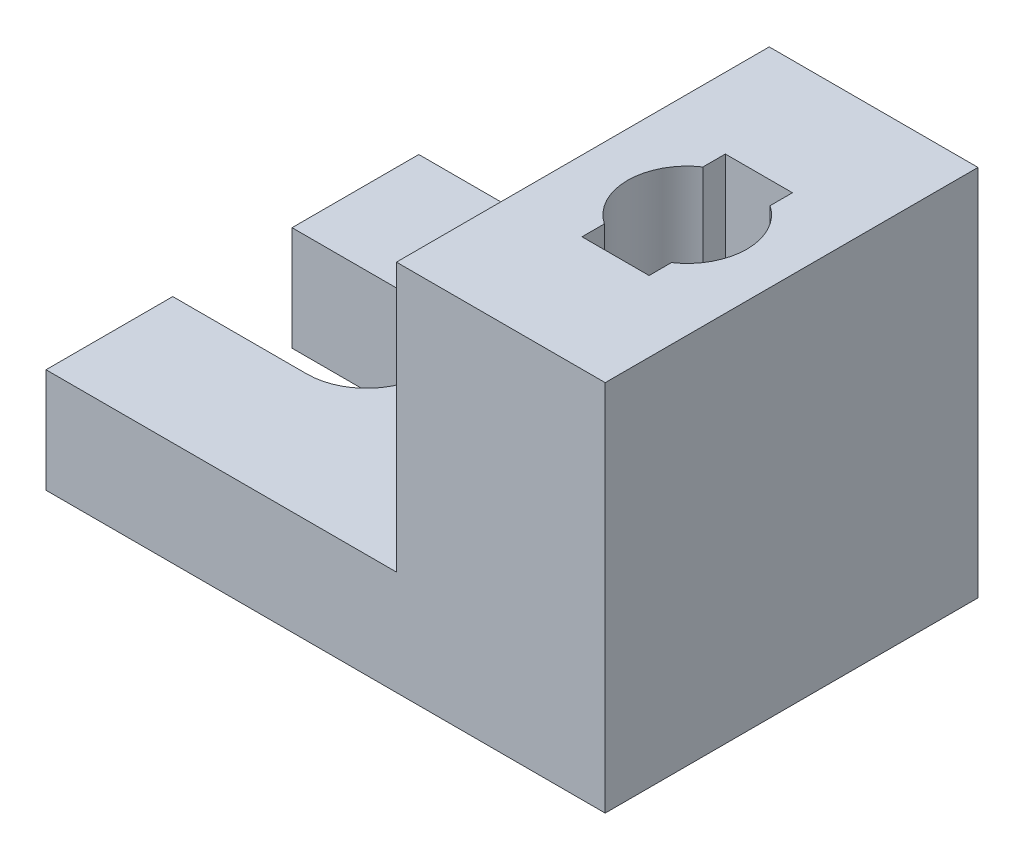
ISO-10303-21;
HEADER;
FILE_DESCRIPTION(('STEP AP214'),'2;1');
FILE_NAME('part.step','',(''),(''),'','','');
FILE_SCHEMA(('AUTOMOTIVE_DESIGN { 1 0 10303 214 1 1 1 1 }'));
ENDSEC;
DATA;
#1=APPLICATION_CONTEXT('core data for automotive mechanical design processes');
#2=APPLICATION_PROTOCOL_DEFINITION('international standard','automotive_design',2000,#1);
#3=PRODUCT_CONTEXT('',#1,'mechanical');
#4=PRODUCT('Part','Part','',(#3));
#5=PRODUCT_RELATED_PRODUCT_CATEGORY('part','',(#4));
#6=PRODUCT_DEFINITION_FORMATION('','',#4);
#7=PRODUCT_DEFINITION_CONTEXT('part definition',#1,'design');
#8=PRODUCT_DEFINITION('design','',#6,#7);
#9=PRODUCT_DEFINITION_SHAPE('','',#8);
#10=(LENGTH_UNIT() NAMED_UNIT(*) SI_UNIT(.MILLI.,.METRE.));
#11=(NAMED_UNIT(*) PLANE_ANGLE_UNIT() SI_UNIT($,.RADIAN.));
#12=(NAMED_UNIT(*) SI_UNIT($,.STERADIAN.) SOLID_ANGLE_UNIT());
#13=UNCERTAINTY_MEASURE_WITH_UNIT(LENGTH_MEASURE(1.E-05),#10,'distance_accuracy_value','');
#14=(GEOMETRIC_REPRESENTATION_CONTEXT(3) GLOBAL_UNCERTAINTY_ASSIGNED_CONTEXT((#13)) GLOBAL_UNIT_ASSIGNED_CONTEXT((#10,
#11,#12)) REPRESENTATION_CONTEXT('',''));
#15=CARTESIAN_POINT('',(0.,0.,0.));
#16=DIRECTION('',(0.,0.,1.));
#17=DIRECTION('',(1.,0.,0.));
#18=AXIS2_PLACEMENT_3D('',#15,#16,#17);
#19=CARTESIAN_POINT('',(0.,0.,100.));
#20=DIRECTION('',(1.,0.,0.));
#21=DIRECTION('',(0.,0.,-1.));
#22=AXIS2_PLACEMENT_3D('',#19,#20,#21);
#23=PLANE('',#22);
#24=DIRECTION('',(0.,0.,-1.));
#25=VECTOR('',#24,1.);
#26=CARTESIAN_POINT('',(0.,28.,100.));
#27=LINE('',#26,#25);
#28=CARTESIAN_POINT('',(0.,28.,100.));
#29=VERTEX_POINT('',#28);
#30=CARTESIAN_POINT('',(0.,28.,66.));
#31=VERTEX_POINT('',#30);
#32=EDGE_CURVE('E335',#29,#31,#27,.T.);
#33=ORIENTED_EDGE('',*,*,#32,.T.);
#34=DIRECTION('',(0.,1.,0.));
#35=VECTOR('',#34,1.);
#36=CARTESIAN_POINT('',(0.,0.,66.));
#37=LINE('',#36,#35);
#38=CARTESIAN_POINT('',(0.,0.,66.));
#39=VERTEX_POINT('',#38);
#40=EDGE_CURVE('E217',#39,#31,#37,.T.);
#41=ORIENTED_EDGE('',*,*,#40,.F.);
#42=DIRECTION('',(0.,0.,-1.));
#43=VECTOR('',#42,1.);
#44=CARTESIAN_POINT('',(0.,0.,100.));
#45=LINE('',#44,#43);
#46=CARTESIAN_POINT('',(0.,0.,100.));
#47=VERTEX_POINT('',#46);
#48=EDGE_CURVE('E11',#47,#39,#45,.T.);
#49=ORIENTED_EDGE('',*,*,#48,.F.);
#50=DIRECTION('',(0.,-1.,0.));
#51=VECTOR('',#50,1.);
#52=CARTESIAN_POINT('',(0.,0.,100.));
#53=LINE('',#52,#51);
#54=EDGE_CURVE('E310',#29,#47,#53,.T.);
#55=ORIENTED_EDGE('',*,*,#54,.F.);
#56=EDGE_LOOP('',(#33,#41,#49,#55));
#57=FACE_BOUND('',#56,.T.);
#58=ADVANCED_FACE('F44',(#57),#23,.F.);
#59=CARTESIAN_POINT('',(56.,28.,40.));
#60=DIRECTION('',(-0.784045824461761,0.620702944365561,0.));
#61=DIRECTION('',(-0.620702944365561,-0.784045824461761,0.));
#62=AXIS2_PLACEMENT_3D('',#59,#60,#61);
#63=PLANE('',#62);
#64=DIRECTION('',(0.620702944365561,0.784045824461761,0.));
#65=VECTOR('',#64,1.);
#66=CARTESIAN_POINT('',(56.,28.,44.));
#67=LINE('',#66,#65);
#68=CARTESIAN_POINT('',(56.,28.,44.));
#69=VERTEX_POINT('',#68);
#70=CARTESIAN_POINT('',(94.,76.,44.));
#71=VERTEX_POINT('',#70);
#72=EDGE_CURVE('E220',#69,#71,#67,.T.);
#73=ORIENTED_EDGE('',*,*,#72,.F.);
#74=DIRECTION('',(0.,0.,1.));
#75=VECTOR('',#74,1.);
#76=CARTESIAN_POINT('',(56.,28.,40.));
#77=LINE('',#76,#75);
#78=CARTESIAN_POINT('',(56.,28.,56.));
#79=VERTEX_POINT('',#78);
#80=EDGE_CURVE('E237',#69,#79,#77,.T.);
#81=ORIENTED_EDGE('',*,*,#80,.T.);
#82=DIRECTION('',(-0.620702944365561,-0.784045824461761,0.));
#83=VECTOR('',#82,1.);
#84=CARTESIAN_POINT('',(56.,28.,56.));
#85=LINE('',#84,#83);
#86=CARTESIAN_POINT('',(94.,76.,56.));
#87=VERTEX_POINT('',#86);
#88=EDGE_CURVE('E226',#87,#79,#85,.T.);
#89=ORIENTED_EDGE('',*,*,#88,.F.);
#90=DIRECTION('',(0.,0.,1.));
#91=VECTOR('',#90,1.);
#92=CARTESIAN_POINT('',(94.,76.,40.));
#93=LINE('',#92,#91);
#94=EDGE_CURVE('E67',#71,#87,#93,.T.);
#95=ORIENTED_EDGE('',*,*,#94,.F.);
#96=EDGE_LOOP('',(#73,#81,#89,#95));
#97=FACE_BOUND('',#96,.T.);
#98=ADVANCED_FACE('F389',(#97),#63,.T.);
#99=CARTESIAN_POINT('',(0.,0.,34.));
#100=VERTEX_POINT('',#99);
#101=CARTESIAN_POINT('',(0.,0.,0.));
#102=VERTEX_POINT('',#101);
#103=EDGE_CURVE('E52',#100,#102,#45,.T.);
#104=ORIENTED_EDGE('',*,*,#103,.F.);
#105=DIRECTION('',(0.,1.,0.));
#106=VECTOR('',#105,1.);
#107=CARTESIAN_POINT('',(0.,0.,34.));
#108=LINE('',#107,#106);
#109=CARTESIAN_POINT('',(0.,28.,34.));
#110=VERTEX_POINT('',#109);
#111=EDGE_CURVE('E193',#100,#110,#108,.T.);
#112=ORIENTED_EDGE('',*,*,#111,.T.);
#113=CARTESIAN_POINT('',(0.,28.,0.));
#114=VERTEX_POINT('',#113);
#115=EDGE_CURVE('E322',#110,#114,#27,.T.);
#116=ORIENTED_EDGE('',*,*,#115,.T.);
#117=DIRECTION('',(0.,-1.,0.));
#118=VECTOR('',#117,1.);
#119=CARTESIAN_POINT('',(0.,0.,0.));
#120=LINE('',#119,#118);
#121=EDGE_CURVE('E292',#114,#102,#120,.T.);
#122=ORIENTED_EDGE('',*,*,#121,.T.);
#123=EDGE_LOOP('',(#104,#112,#116,#122));
#124=FACE_BOUND('',#123,.T.);
#125=ADVANCED_FACE('F50',(#124),#23,.F.);
#126=CARTESIAN_POINT('',(0.,0.,100.));
#127=DIRECTION('',(0.,1.,0.));
#128=DIRECTION('',(0.,0.,1.));
#129=AXIS2_PLACEMENT_3D('',#126,#127,#128);
#130=PLANE('',#129);
#131=ORIENTED_EDGE('',*,*,#48,.T.);
#132=DIRECTION('',(1.,0.,0.));
#133=VECTOR('',#132,1.);
#134=CARTESIAN_POINT('',(36.,0.,66.));
#135=LINE('',#134,#133);
#136=CARTESIAN_POINT('',(36.,0.,66.));
#137=VERTEX_POINT('',#136);
#138=EDGE_CURVE('E196',#39,#137,#135,.T.);
#139=ORIENTED_EDGE('',*,*,#138,.T.);
#140=CARTESIAN_POINT('',(36.,0.,50.));
#141=DIRECTION('',(0.,1.,0.));
#142=DIRECTION('',(0.,0.,1.));
#143=AXIS2_PLACEMENT_3D('',#140,#141,#142);
#144=CIRCLE('',#143,16.);
#145=CARTESIAN_POINT('',(36.,0.,34.));
#146=VERTEX_POINT('',#145);
#147=EDGE_CURVE('E192',#137,#146,#144,.T.);
#148=ORIENTED_EDGE('',*,*,#147,.T.);
#149=DIRECTION('',(-1.,0.,0.));
#150=VECTOR('',#149,1.);
#151=CARTESIAN_POINT('',(36.,0.,34.));
#152=LINE('',#151,#150);
#153=EDGE_CURVE('E198',#146,#100,#152,.T.);
#154=ORIENTED_EDGE('',*,*,#153,.T.);
#155=ORIENTED_EDGE('',*,*,#103,.T.);
#156=DIRECTION('',(1.,0.,0.));
#157=VECTOR('',#156,1.);
#158=CARTESIAN_POINT('',(0.,0.,0.));
#159=LINE('',#158,#157);
#160=CARTESIAN_POINT('',(150.,0.,0.));
#161=VERTEX_POINT('',#160);
#162=EDGE_CURVE('E321',#102,#161,#159,.T.);
#163=ORIENTED_EDGE('',*,*,#162,.T.);
#164=DIRECTION('',(0.,0.,-1.));
#165=VECTOR('',#164,1.);
#166=CARTESIAN_POINT('',(150.,0.,100.));
#167=LINE('',#166,#165);
#168=CARTESIAN_POINT('',(150.,0.,100.));
#169=VERTEX_POINT('',#168);
#170=EDGE_CURVE('E343',#169,#161,#167,.T.);
#171=ORIENTED_EDGE('',*,*,#170,.F.);
#172=DIRECTION('',(1.,0.,0.));
#173=VECTOR('',#172,1.);
#174=CARTESIAN_POINT('',(0.,0.,100.));
#175=LINE('',#174,#173);
#176=EDGE_CURVE('E309',#47,#169,#175,.T.);
#177=ORIENTED_EDGE('',*,*,#176,.F.);
#178=EDGE_LOOP('',(#131,#139,#148,#154,#155,#163,#171,#177));
#179=FACE_BOUND('',#178,.T.);
#180=ADVANCED_FACE('F205',(#179),#130,.F.);
#181=CARTESIAN_POINT('',(150.,0.,100.));
#182=DIRECTION('',(-1.,0.,0.));
#183=DIRECTION('',(0.,0.,1.));
#184=AXIS2_PLACEMENT_3D('',#181,#182,#183);
#185=PLANE('',#184);
#186=DIRECTION('',(0.,1.,0.));
#187=VECTOR('',#186,1.);
#188=CARTESIAN_POINT('',(150.,0.,0.));
#189=LINE('',#188,#187);
#190=CARTESIAN_POINT('',(150.,100.,0.));
#191=VERTEX_POINT('',#190);
#192=EDGE_CURVE('E326',#161,#191,#189,.T.);
#193=ORIENTED_EDGE('',*,*,#192,.T.);
#194=DIRECTION('',(0.,0.,-1.));
#195=VECTOR('',#194,1.);
#196=CARTESIAN_POINT('',(150.,100.,100.));
#197=LINE('',#196,#195);
#198=CARTESIAN_POINT('',(150.,100.,100.));
#199=VERTEX_POINT('',#198);
#200=EDGE_CURVE('E344',#199,#191,#197,.T.);
#201=ORIENTED_EDGE('',*,*,#200,.F.);
#202=DIRECTION('',(0.,1.,0.));
#203=VECTOR('',#202,1.);
#204=CARTESIAN_POINT('',(150.,0.,100.));
#205=LINE('',#204,#203);
#206=EDGE_CURVE('E312',#169,#199,#205,.T.);
#207=ORIENTED_EDGE('',*,*,#206,.F.);
#208=ORIENTED_EDGE('',*,*,#170,.T.);
#209=EDGE_LOOP('',(#193,#201,#207,#208));
#210=FACE_BOUND('',#209,.T.);
#211=ADVANCED_FACE('F369',(#210),#185,.F.);
#212=CARTESIAN_POINT('',(150.,100.,100.));
#213=DIRECTION('',(0.,-1.,0.));
#214=DIRECTION('',(0.,0.,-1.));
#215=AXIS2_PLACEMENT_3D('',#212,#213,#214);
#216=PLANE('',#215);
#217=DIRECTION('',(0.,0.,-1.));
#218=VECTOR('',#217,1.);
#219=CARTESIAN_POINT('',(131.,100.,30.7712434446771));
#220=LINE('',#219,#218);
#221=CARTESIAN_POINT('',(131.,100.,36.7712434446771));
#222=VERTEX_POINT('',#221);
#223=CARTESIAN_POINT('',(131.,100.,30.7712434446771));
#224=VERTEX_POINT('',#223);
#225=EDGE_CURVE('E270',#222,#224,#220,.T.);
#226=ORIENTED_EDGE('',*,*,#225,.F.);
#227=CARTESIAN_POINT('',(122.,100.,50.));
#228=DIRECTION('',(0.,1.,0.));
#229=DIRECTION('',(0.,0.,1.));
#230=AXIS2_PLACEMENT_3D('',#227,#228,#229);
#231=CIRCLE('',#230,16.);
#232=CARTESIAN_POINT('',(131.,100.,63.2287565553229));
#233=VERTEX_POINT('',#232);
#234=EDGE_CURVE('E241',#233,#222,#231,.T.);
#235=ORIENTED_EDGE('',*,*,#234,.F.);
#236=DIRECTION('',(0.,0.,-1.));
#237=VECTOR('',#236,1.);
#238=CARTESIAN_POINT('',(131.,100.,63.2287565553229));
#239=LINE('',#238,#237);
#240=CARTESIAN_POINT('',(131.,100.,69.2287565553229));
#241=VERTEX_POINT('',#240);
#242=EDGE_CURVE('E250',#241,#233,#239,.T.);
#243=ORIENTED_EDGE('',*,*,#242,.F.);
#244=DIRECTION('',(1.,0.,0.));
#245=VECTOR('',#244,1.);
#246=CARTESIAN_POINT('',(113.,100.,69.228756555323));
#247=LINE('',#246,#245);
#248=CARTESIAN_POINT('',(113.,100.,69.228756555323));
#249=VERTEX_POINT('',#248);
#250=EDGE_CURVE('E284',#249,#241,#247,.T.);
#251=ORIENTED_EDGE('',*,*,#250,.F.);
#252=DIRECTION('',(0.,0.,1.));
#253=VECTOR('',#252,1.);
#254=CARTESIAN_POINT('',(113.,100.,63.228756555323));
#255=LINE('',#254,#253);
#256=CARTESIAN_POINT('',(113.,100.,63.228756555323));
#257=VERTEX_POINT('',#256);
#258=EDGE_CURVE('E285',#257,#249,#255,.T.);
#259=ORIENTED_EDGE('',*,*,#258,.F.);
#260=CARTESIAN_POINT('',(122.,100.,50.));
#261=DIRECTION('',(0.,1.,0.));
#262=DIRECTION('',(0.,0.,1.));
#263=AXIS2_PLACEMENT_3D('',#260,#261,#262);
#264=CIRCLE('',#263,16.);
#265=CARTESIAN_POINT('',(113.,100.,36.7712434446771));
#266=VERTEX_POINT('',#265);
#267=EDGE_CURVE('E276',#266,#257,#264,.T.);
#268=ORIENTED_EDGE('',*,*,#267,.F.);
#269=DIRECTION('',(0.,0.,1.));
#270=VECTOR('',#269,1.);
#271=CARTESIAN_POINT('',(113.,100.,30.7712434446771));
#272=LINE('',#271,#270);
#273=CARTESIAN_POINT('',(113.,100.,30.7712434446771));
#274=VERTEX_POINT('',#273);
#275=EDGE_CURVE('E277',#274,#266,#272,.T.);
#276=ORIENTED_EDGE('',*,*,#275,.F.);
#277=DIRECTION('',(-1.,0.,0.));
#278=VECTOR('',#277,1.);
#279=CARTESIAN_POINT('',(113.,100.,30.7712434446771));
#280=LINE('',#279,#278);
#281=EDGE_CURVE('E271',#224,#274,#280,.T.);
#282=ORIENTED_EDGE('',*,*,#281,.F.);
#283=EDGE_LOOP('',(#226,#235,#243,#251,#259,#268,#276,#282));
#284=FACE_BOUND('',#283,.T.);
#285=DIRECTION('',(-1.,0.,0.));
#286=VECTOR('',#285,1.);
#287=CARTESIAN_POINT('',(150.,100.,0.));
#288=LINE('',#287,#286);
#289=CARTESIAN_POINT('',(94.,100.,0.));
#290=VERTEX_POINT('',#289);
#291=EDGE_CURVE('E327',#191,#290,#288,.T.);
#292=ORIENTED_EDGE('',*,*,#291,.T.);
#293=DIRECTION('',(0.,0.,-1.));
#294=VECTOR('',#293,1.);
#295=CARTESIAN_POINT('',(94.,100.,100.));
#296=LINE('',#295,#294);
#297=CARTESIAN_POINT('',(94.,100.,100.));
#298=VERTEX_POINT('',#297);
#299=EDGE_CURVE('E338',#298,#290,#296,.T.);
#300=ORIENTED_EDGE('',*,*,#299,.F.);
#301=DIRECTION('',(-1.,0.,0.));
#302=VECTOR('',#301,1.);
#303=CARTESIAN_POINT('',(150.,100.,100.));
#304=LINE('',#303,#302);
#305=EDGE_CURVE('E314',#199,#298,#304,.T.);
#306=ORIENTED_EDGE('',*,*,#305,.F.);
#307=ORIENTED_EDGE('',*,*,#200,.T.);
#308=EDGE_LOOP('',(#292,#300,#306,#307));
#309=FACE_BOUND('',#308,.T.);
#310=ADVANCED_FACE('F368',(#284,#309),#216,.F.);
#311=CARTESIAN_POINT('',(94.,28.,100.));
#312=DIRECTION('',(1.,0.,0.));
#313=DIRECTION('',(0.,0.,-1.));
#314=AXIS2_PLACEMENT_3D('',#311,#312,#313);
#315=PLANE('',#314);
#316=DIRECTION('',(0.,-1.,0.));
#317=VECTOR('',#316,1.);
#318=CARTESIAN_POINT('',(94.,76.,44.));
#319=LINE('',#318,#317);
#320=CARTESIAN_POINT('',(94.,28.,44.));
#321=VERTEX_POINT('',#320);
#322=EDGE_CURVE('E224',#71,#321,#319,.T.);
#323=ORIENTED_EDGE('',*,*,#322,.F.);
#324=ORIENTED_EDGE('',*,*,#94,.T.);
#325=DIRECTION('',(0.,1.,0.));
#326=VECTOR('',#325,1.);
#327=CARTESIAN_POINT('',(94.,76.,56.));
#328=LINE('',#327,#326);
#329=CARTESIAN_POINT('',(94.,28.,56.));
#330=VERTEX_POINT('',#329);
#331=EDGE_CURVE('E234',#330,#87,#328,.T.);
#332=ORIENTED_EDGE('',*,*,#331,.F.);
#333=DIRECTION('',(0.,0.,1.));
#334=VECTOR('',#333,1.);
#335=CARTESIAN_POINT('',(94.,28.,56.));
#336=LINE('',#335,#334);
#337=CARTESIAN_POINT('',(94.,28.,100.));
#338=VERTEX_POINT('',#337);
#339=EDGE_CURVE('E236',#330,#338,#336,.T.);
#340=ORIENTED_EDGE('',*,*,#339,.T.);
#341=DIRECTION('',(0.,-1.,0.));
#342=VECTOR('',#341,1.);
#343=CARTESIAN_POINT('',(94.,28.,100.));
#344=LINE('',#343,#342);
#345=EDGE_CURVE('E320',#298,#338,#344,.T.);
#346=ORIENTED_EDGE('',*,*,#345,.F.);
#347=ORIENTED_EDGE('',*,*,#299,.T.);
#348=DIRECTION('',(0.,-1.,0.));
#349=VECTOR('',#348,1.);
#350=CARTESIAN_POINT('',(94.,28.,0.));
#351=LINE('',#350,#349);
#352=CARTESIAN_POINT('',(94.,28.,0.));
#353=VERTEX_POINT('',#352);
#354=EDGE_CURVE('E329',#290,#353,#351,.T.);
#355=ORIENTED_EDGE('',*,*,#354,.T.);
#356=DIRECTION('',(0.,0.,-1.));
#357=VECTOR('',#356,1.);
#358=CARTESIAN_POINT('',(94.,28.,100.));
#359=LINE('',#358,#357);
#360=EDGE_CURVE('E336',#321,#353,#359,.T.);
#361=ORIENTED_EDGE('',*,*,#360,.F.);
#362=EDGE_LOOP('',(#323,#324,#332,#340,#346,#347,#355,#361));
#363=FACE_BOUND('',#362,.T.);
#364=ADVANCED_FACE('F361',(#363),#315,.F.);
#365=CARTESIAN_POINT('',(0.,28.,100.));
#366=DIRECTION('',(0.,-1.,0.));
#367=DIRECTION('',(0.,0.,-1.));
#368=AXIS2_PLACEMENT_3D('',#365,#366,#367);
#369=PLANE('',#368);
#370=CARTESIAN_POINT('',(36.,28.,50.));
#371=DIRECTION('',(0.,1.,0.));
#372=DIRECTION('',(0.,0.,1.));
#373=AXIS2_PLACEMENT_3D('',#370,#371,#372);
#374=CIRCLE('',#373,16.);
#375=CARTESIAN_POINT('',(36.,28.,66.));
#376=VERTEX_POINT('',#375);
#377=CARTESIAN_POINT('',(36.,28.,34.));
#378=VERTEX_POINT('',#377);
#379=EDGE_CURVE('E58',#376,#378,#374,.T.);
#380=ORIENTED_EDGE('',*,*,#379,.F.);
#381=DIRECTION('',(1.,0.,0.));
#382=VECTOR('',#381,1.);
#383=CARTESIAN_POINT('',(36.,28.,66.));
#384=LINE('',#383,#382);
#385=EDGE_CURVE('E207',#31,#376,#384,.T.);
#386=ORIENTED_EDGE('',*,*,#385,.F.);
#387=ORIENTED_EDGE('',*,*,#32,.F.);
#388=DIRECTION('',(-1.,0.,0.));
#389=VECTOR('',#388,1.);
#390=CARTESIAN_POINT('',(0.,28.,100.));
#391=LINE('',#390,#389);
#392=EDGE_CURVE('E316',#338,#29,#391,.T.);
#393=ORIENTED_EDGE('',*,*,#392,.F.);
#394=ORIENTED_EDGE('',*,*,#339,.F.);
#395=DIRECTION('',(1.,0.,0.));
#396=VECTOR('',#395,1.);
#397=CARTESIAN_POINT('',(94.,28.,56.));
#398=LINE('',#397,#396);
#399=EDGE_CURVE('E233',#79,#330,#398,.T.);
#400=ORIENTED_EDGE('',*,*,#399,.F.);
#401=ORIENTED_EDGE('',*,*,#80,.F.);
#402=DIRECTION('',(-1.,0.,0.));
#403=VECTOR('',#402,1.);
#404=CARTESIAN_POINT('',(94.,28.,44.));
#405=LINE('',#404,#403);
#406=EDGE_CURVE('E228',#321,#69,#405,.T.);
#407=ORIENTED_EDGE('',*,*,#406,.F.);
#408=ORIENTED_EDGE('',*,*,#360,.T.);
#409=DIRECTION('',(-1.,0.,0.));
#410=VECTOR('',#409,1.);
#411=CARTESIAN_POINT('',(0.,28.,0.));
#412=LINE('',#411,#410);
#413=EDGE_CURVE('E311',#353,#114,#412,.T.);
#414=ORIENTED_EDGE('',*,*,#413,.T.);
#415=ORIENTED_EDGE('',*,*,#115,.F.);
#416=DIRECTION('',(-1.,0.,0.));
#417=VECTOR('',#416,1.);
#418=CARTESIAN_POINT('',(36.,28.,34.));
#419=LINE('',#418,#417);
#420=EDGE_CURVE('E209',#378,#110,#419,.T.);
#421=ORIENTED_EDGE('',*,*,#420,.F.);
#422=EDGE_LOOP('',(#380,#386,#387,#393,#394,#400,#401,#407,#408,#414,#415,#421));
#423=FACE_BOUND('',#422,.T.);
#424=ADVANCED_FACE('F359',(#423),#369,.F.);
#425=CARTESIAN_POINT('',(0.,0.,100.));
#426=DIRECTION('',(0.,0.,-1.));
#427=DIRECTION('',(-1.,0.,0.));
#428=AXIS2_PLACEMENT_3D('',#425,#426,#427);
#429=PLANE('',#428);
#430=ORIENTED_EDGE('',*,*,#345,.T.);
#431=ORIENTED_EDGE('',*,*,#392,.T.);
#432=ORIENTED_EDGE('',*,*,#54,.T.);
#433=ORIENTED_EDGE('',*,*,#176,.T.);
#434=ORIENTED_EDGE('',*,*,#206,.T.);
#435=ORIENTED_EDGE('',*,*,#305,.T.);
#436=EDGE_LOOP('',(#430,#431,#432,#433,#434,#435));
#437=FACE_BOUND('',#436,.T.);
#438=ADVANCED_FACE('F375',(#437),#429,.F.);
#439=CARTESIAN_POINT('',(0.,0.,0.));
#440=DIRECTION('',(0.,0.,-1.));
#441=DIRECTION('',(-1.,0.,0.));
#442=AXIS2_PLACEMENT_3D('',#439,#440,#441);
#443=PLANE('',#442);
#444=ORIENTED_EDGE('',*,*,#121,.F.);
#445=ORIENTED_EDGE('',*,*,#413,.F.);
#446=ORIENTED_EDGE('',*,*,#354,.F.);
#447=ORIENTED_EDGE('',*,*,#291,.F.);
#448=ORIENTED_EDGE('',*,*,#192,.F.);
#449=ORIENTED_EDGE('',*,*,#162,.F.);
#450=EDGE_LOOP('',(#444,#445,#446,#447,#448,#449));
#451=FACE_BOUND('',#450,.T.);
#452=ADVANCED_FACE('F355',(#451),#443,.T.);
#453=CARTESIAN_POINT('',(122.,50.,50.));
#454=DIRECTION('',(0.,1.,0.));
#455=DIRECTION('',(0.,0.,1.));
#456=AXIS2_PLACEMENT_3D('',#453,#454,#455);
#457=CYLINDRICAL_SURFACE('',#456,16.);
#458=ORIENTED_EDGE('',*,*,#234,.T.);
#459=DIRECTION('',(0.,1.,0.));
#460=VECTOR('',#459,1.);
#461=CARTESIAN_POINT('',(131.,50.,36.7712434446771));
#462=LINE('',#461,#460);
#463=CARTESIAN_POINT('',(131.,50.,36.7712434446771));
#464=VERTEX_POINT('',#463);
#465=EDGE_CURVE('E269',#464,#222,#462,.T.);
#466=ORIENTED_EDGE('',*,*,#465,.F.);
#467=CARTESIAN_POINT('',(122.,50.,50.));
#468=DIRECTION('',(0.,1.,0.));
#469=DIRECTION('',(0.,0.,1.));
#470=AXIS2_PLACEMENT_3D('',#467,#468,#469);
#471=CIRCLE('',#470,16.);
#472=CARTESIAN_POINT('',(131.,50.,63.2287565553229));
#473=VERTEX_POINT('',#472);
#474=EDGE_CURVE('E243',#473,#464,#471,.T.);
#475=ORIENTED_EDGE('',*,*,#474,.F.);
#476=DIRECTION('',(0.,1.,0.));
#477=VECTOR('',#476,1.);
#478=CARTESIAN_POINT('',(131.,50.,63.2287565553229));
#479=LINE('',#478,#477);
#480=EDGE_CURVE('E290',#473,#233,#479,.T.);
#481=ORIENTED_EDGE('',*,*,#480,.T.);
#482=EDGE_LOOP('',(#458,#466,#475,#481));
#483=FACE_BOUND('',#482,.T.);
#484=ADVANCED_FACE('F424',(#483),#457,.F.);
#485=CARTESIAN_POINT('',(131.,50.,63.2287565553229));
#486=DIRECTION('',(1.,0.,0.));
#487=DIRECTION('',(0.,0.,-1.));
#488=AXIS2_PLACEMENT_3D('',#485,#486,#487);
#489=PLANE('',#488);
#490=ORIENTED_EDGE('',*,*,#242,.T.);
#491=ORIENTED_EDGE('',*,*,#480,.F.);
#492=DIRECTION('',(0.,0.,-1.));
#493=VECTOR('',#492,1.);
#494=CARTESIAN_POINT('',(131.,50.,63.2287565553229));
#495=LINE('',#494,#493);
#496=CARTESIAN_POINT('',(131.,50.,69.2287565553229));
#497=VERTEX_POINT('',#496);
#498=EDGE_CURVE('E264',#497,#473,#495,.T.);
#499=ORIENTED_EDGE('',*,*,#498,.F.);
#500=DIRECTION('',(0.,1.,0.));
#501=VECTOR('',#500,1.);
#502=CARTESIAN_POINT('',(131.,50.,69.2287565553229));
#503=LINE('',#502,#501);
#504=EDGE_CURVE('E291',#497,#241,#503,.T.);
#505=ORIENTED_EDGE('',*,*,#504,.T.);
#506=EDGE_LOOP('',(#490,#491,#499,#505));
#507=FACE_BOUND('',#506,.T.);
#508=ADVANCED_FACE('F427',(#507),#489,.F.);
#509=CARTESIAN_POINT('',(113.,50.,69.228756555323));
#510=DIRECTION('',(0.,0.,1.));
#511=DIRECTION('',(1.,0.,0.));
#512=AXIS2_PLACEMENT_3D('',#509,#510,#511);
#513=PLANE('',#512);
#514=ORIENTED_EDGE('',*,*,#250,.T.);
#515=ORIENTED_EDGE('',*,*,#504,.F.);
#516=DIRECTION('',(1.,0.,0.));
#517=VECTOR('',#516,1.);
#518=CARTESIAN_POINT('',(113.,50.,69.228756555323));
#519=LINE('',#518,#517);
#520=CARTESIAN_POINT('',(113.,50.,69.228756555323));
#521=VERTEX_POINT('',#520);
#522=EDGE_CURVE('E265',#521,#497,#519,.T.);
#523=ORIENTED_EDGE('',*,*,#522,.F.);
#524=DIRECTION('',(0.,1.,0.));
#525=VECTOR('',#524,1.);
#526=CARTESIAN_POINT('',(113.,50.,69.228756555323));
#527=LINE('',#526,#525);
#528=EDGE_CURVE('E294',#521,#249,#527,.T.);
#529=ORIENTED_EDGE('',*,*,#528,.T.);
#530=EDGE_LOOP('',(#514,#515,#523,#529));
#531=FACE_BOUND('',#530,.T.);
#532=ADVANCED_FACE('F452',(#531),#513,.F.);
#533=CARTESIAN_POINT('',(113.,50.,63.228756555323));
#534=DIRECTION('',(-1.,0.,0.));
#535=DIRECTION('',(0.,0.,1.));
#536=AXIS2_PLACEMENT_3D('',#533,#534,#535);
#537=PLANE('',#536);
#538=ORIENTED_EDGE('',*,*,#258,.T.);
#539=ORIENTED_EDGE('',*,*,#528,.F.);
#540=DIRECTION('',(0.,0.,1.));
#541=VECTOR('',#540,1.);
#542=CARTESIAN_POINT('',(113.,50.,63.228756555323));
#543=LINE('',#542,#541);
#544=CARTESIAN_POINT('',(113.,50.,63.228756555323));
#545=VERTEX_POINT('',#544);
#546=EDGE_CURVE('E256',#545,#521,#543,.T.);
#547=ORIENTED_EDGE('',*,*,#546,.F.);
#548=DIRECTION('',(0.,1.,0.));
#549=VECTOR('',#548,1.);
#550=CARTESIAN_POINT('',(113.,50.,63.228756555323));
#551=LINE('',#550,#549);
#552=EDGE_CURVE('E300',#545,#257,#551,.T.);
#553=ORIENTED_EDGE('',*,*,#552,.T.);
#554=EDGE_LOOP('',(#538,#539,#547,#553));
#555=FACE_BOUND('',#554,.T.);
#556=ADVANCED_FACE('F450',(#555),#537,.F.);
#557=CARTESIAN_POINT('',(122.,50.,50.));
#558=DIRECTION('',(0.,1.,0.));
#559=DIRECTION('',(0.,0.,1.));
#560=AXIS2_PLACEMENT_3D('',#557,#558,#559);
#561=CYLINDRICAL_SURFACE('',#560,16.);
#562=ORIENTED_EDGE('',*,*,#267,.T.);
#563=ORIENTED_EDGE('',*,*,#552,.F.);
#564=CARTESIAN_POINT('',(122.,50.,50.));
#565=DIRECTION('',(0.,1.,0.));
#566=DIRECTION('',(0.,0.,1.));
#567=AXIS2_PLACEMENT_3D('',#564,#565,#566);
#568=CIRCLE('',#567,16.);
#569=CARTESIAN_POINT('',(113.,50.,36.7712434446771));
#570=VERTEX_POINT('',#569);
#571=EDGE_CURVE('E257',#570,#545,#568,.T.);
#572=ORIENTED_EDGE('',*,*,#571,.F.);
#573=DIRECTION('',(0.,1.,0.));
#574=VECTOR('',#573,1.);
#575=CARTESIAN_POINT('',(113.,50.,36.7712434446771));
#576=LINE('',#575,#574);
#577=EDGE_CURVE('E299',#570,#266,#576,.T.);
#578=ORIENTED_EDGE('',*,*,#577,.T.);
#579=EDGE_LOOP('',(#562,#563,#572,#578));
#580=FACE_BOUND('',#579,.T.);
#581=ADVANCED_FACE('F442',(#580),#561,.F.);
#582=CARTESIAN_POINT('',(113.,50.,30.7712434446771));
#583=DIRECTION('',(-1.,0.,0.));
#584=DIRECTION('',(0.,0.,1.));
#585=AXIS2_PLACEMENT_3D('',#582,#583,#584);
#586=PLANE('',#585);
#587=ORIENTED_EDGE('',*,*,#275,.T.);
#588=ORIENTED_EDGE('',*,*,#577,.F.);
#589=DIRECTION('',(0.,0.,1.));
#590=VECTOR('',#589,1.);
#591=CARTESIAN_POINT('',(113.,50.,30.7712434446771));
#592=LINE('',#591,#590);
#593=CARTESIAN_POINT('',(113.,50.,30.7712434446771));
#594=VERTEX_POINT('',#593);
#595=EDGE_CURVE('E254',#594,#570,#592,.T.);
#596=ORIENTED_EDGE('',*,*,#595,.F.);
#597=DIRECTION('',(0.,1.,0.));
#598=VECTOR('',#597,1.);
#599=CARTESIAN_POINT('',(113.,50.,30.7712434446771));
#600=LINE('',#599,#598);
#601=EDGE_CURVE('E301',#594,#274,#600,.T.);
#602=ORIENTED_EDGE('',*,*,#601,.T.);
#603=EDGE_LOOP('',(#587,#588,#596,#602));
#604=FACE_BOUND('',#603,.T.);
#605=ADVANCED_FACE('F437',(#604),#586,.F.);
#606=CARTESIAN_POINT('',(113.,50.,30.7712434446771));
#607=DIRECTION('',(0.,0.,-1.));
#608=DIRECTION('',(-1.,0.,0.));
#609=AXIS2_PLACEMENT_3D('',#606,#607,#608);
#610=PLANE('',#609);
#611=ORIENTED_EDGE('',*,*,#281,.T.);
#612=ORIENTED_EDGE('',*,*,#601,.F.);
#613=DIRECTION('',(-1.,0.,0.));
#614=VECTOR('',#613,1.);
#615=CARTESIAN_POINT('',(113.,50.,30.7712434446771));
#616=LINE('',#615,#614);
#617=CARTESIAN_POINT('',(131.,50.,30.7712434446771));
#618=VERTEX_POINT('',#617);
#619=EDGE_CURVE('E249',#618,#594,#616,.T.);
#620=ORIENTED_EDGE('',*,*,#619,.F.);
#621=DIRECTION('',(0.,1.,0.));
#622=VECTOR('',#621,1.);
#623=CARTESIAN_POINT('',(131.,50.,30.7712434446771));
#624=LINE('',#623,#622);
#625=EDGE_CURVE('E303',#618,#224,#624,.T.);
#626=ORIENTED_EDGE('',*,*,#625,.T.);
#627=EDGE_LOOP('',(#611,#612,#620,#626));
#628=FACE_BOUND('',#627,.T.);
#629=ADVANCED_FACE('F434',(#628),#610,.F.);
#630=CARTESIAN_POINT('',(131.,50.,30.7712434446771));
#631=DIRECTION('',(1.,0.,0.));
#632=DIRECTION('',(0.,0.,-1.));
#633=AXIS2_PLACEMENT_3D('',#630,#631,#632);
#634=PLANE('',#633);
#635=ORIENTED_EDGE('',*,*,#225,.T.);
#636=ORIENTED_EDGE('',*,*,#625,.F.);
#637=DIRECTION('',(0.,0.,-1.));
#638=VECTOR('',#637,1.);
#639=CARTESIAN_POINT('',(131.,50.,30.7712434446771));
#640=LINE('',#639,#638);
#641=EDGE_CURVE('E246',#464,#618,#640,.T.);
#642=ORIENTED_EDGE('',*,*,#641,.F.);
#643=ORIENTED_EDGE('',*,*,#465,.T.);
#644=EDGE_LOOP('',(#635,#636,#642,#643));
#645=FACE_BOUND('',#644,.T.);
#646=ADVANCED_FACE('F435',(#645),#634,.F.);
#647=CARTESIAN_POINT('',(122.,50.,50.));
#648=DIRECTION('',(0.,1.,0.));
#649=DIRECTION('',(0.,0.,1.));
#650=AXIS2_PLACEMENT_3D('',#647,#648,#649);
#651=PLANE('',#650);
#652=ORIENTED_EDGE('',*,*,#474,.T.);
#653=ORIENTED_EDGE('',*,*,#641,.T.);
#654=ORIENTED_EDGE('',*,*,#619,.T.);
#655=ORIENTED_EDGE('',*,*,#595,.T.);
#656=ORIENTED_EDGE('',*,*,#571,.T.);
#657=ORIENTED_EDGE('',*,*,#546,.T.);
#658=ORIENTED_EDGE('',*,*,#522,.T.);
#659=ORIENTED_EDGE('',*,*,#498,.T.);
#660=EDGE_LOOP('',(#652,#653,#654,#655,#656,#657,#658,#659));
#661=FACE_BOUND('',#660,.T.);
#662=ADVANCED_FACE('F398',(#661),#651,.T.);
#663=CARTESIAN_POINT('',(0.,0.,56.));
#664=DIRECTION('',(0.,0.,1.));
#665=DIRECTION('',(1.,0.,0.));
#666=AXIS2_PLACEMENT_3D('',#663,#664,#665);
#667=PLANE('',#666);
#668=ORIENTED_EDGE('',*,*,#88,.T.);
#669=ORIENTED_EDGE('',*,*,#399,.T.);
#670=ORIENTED_EDGE('',*,*,#331,.T.);
#671=EDGE_LOOP('',(#668,#669,#670));
#672=FACE_BOUND('',#671,.T.);
#673=ADVANCED_FACE('F383',(#672),#667,.T.);
#674=CARTESIAN_POINT('',(0.,0.,44.));
#675=DIRECTION('',(0.,0.,1.));
#676=DIRECTION('',(1.,0.,0.));
#677=AXIS2_PLACEMENT_3D('',#674,#675,#676);
#678=PLANE('',#677);
#679=ORIENTED_EDGE('',*,*,#72,.T.);
#680=ORIENTED_EDGE('',*,*,#322,.T.);
#681=ORIENTED_EDGE('',*,*,#406,.T.);
#682=EDGE_LOOP('',(#679,#680,#681));
#683=FACE_BOUND('',#682,.T.);
#684=ADVANCED_FACE('F391',(#683),#678,.F.);
#685=CARTESIAN_POINT('',(36.,0.,50.));
#686=DIRECTION('',(0.,1.,0.));
#687=DIRECTION('',(0.,0.,1.));
#688=AXIS2_PLACEMENT_3D('',#685,#686,#687);
#689=CYLINDRICAL_SURFACE('',#688,16.);
#690=ORIENTED_EDGE('',*,*,#379,.T.);
#691=DIRECTION('',(0.,1.,0.));
#692=VECTOR('',#691,1.);
#693=CARTESIAN_POINT('',(36.,0.,34.));
#694=LINE('',#693,#692);
#695=EDGE_CURVE('E190',#146,#378,#694,.T.);
#696=ORIENTED_EDGE('',*,*,#695,.F.);
#697=ORIENTED_EDGE('',*,*,#147,.F.);
#698=DIRECTION('',(0.,1.,0.));
#699=VECTOR('',#698,1.);
#700=CARTESIAN_POINT('',(36.,0.,66.));
#701=LINE('',#700,#699);
#702=EDGE_CURVE('E213',#137,#376,#701,.T.);
#703=ORIENTED_EDGE('',*,*,#702,.T.);
#704=EDGE_LOOP('',(#690,#696,#697,#703));
#705=FACE_BOUND('',#704,.T.);
#706=ADVANCED_FACE('F186',(#705),#689,.F.);
#707=CARTESIAN_POINT('',(36.,0.,66.));
#708=DIRECTION('',(0.,0.,1.));
#709=DIRECTION('',(1.,0.,0.));
#710=AXIS2_PLACEMENT_3D('',#707,#708,#709);
#711=PLANE('',#710);
#712=ORIENTED_EDGE('',*,*,#385,.T.);
#713=ORIENTED_EDGE('',*,*,#702,.F.);
#714=ORIENTED_EDGE('',*,*,#138,.F.);
#715=ORIENTED_EDGE('',*,*,#40,.T.);
#716=EDGE_LOOP('',(#712,#713,#714,#715));
#717=FACE_BOUND('',#716,.T.);
#718=ADVANCED_FACE('F379',(#717),#711,.F.);
#719=CARTESIAN_POINT('',(36.,0.,34.));
#720=DIRECTION('',(0.,0.,-1.));
#721=DIRECTION('',(-1.,0.,0.));
#722=AXIS2_PLACEMENT_3D('',#719,#720,#721);
#723=PLANE('',#722);
#724=ORIENTED_EDGE('',*,*,#420,.T.);
#725=ORIENTED_EDGE('',*,*,#111,.F.);
#726=ORIENTED_EDGE('',*,*,#153,.F.);
#727=ORIENTED_EDGE('',*,*,#695,.T.);
#728=EDGE_LOOP('',(#724,#725,#726,#727));
#729=FACE_BOUND('',#728,.T.);
#730=ADVANCED_FACE('F199',(#729),#723,.F.);
#731=CLOSED_SHELL('',(#58,#98,#125,#180,#211,#310,#364,#424,#438,#452,#484,#508,#532,#556,#581,
#605,#629,#646,#662,#673,#684,#706,#718,#730));
#732=MANIFOLD_SOLID_BREP('B2',#731);
#733=ADVANCED_BREP_SHAPE_REPRESENTATION('',(#18,#732),#14);
#734=SHAPE_DEFINITION_REPRESENTATION(#9,#733);
ENDSEC;
END-ISO-10303-21;
